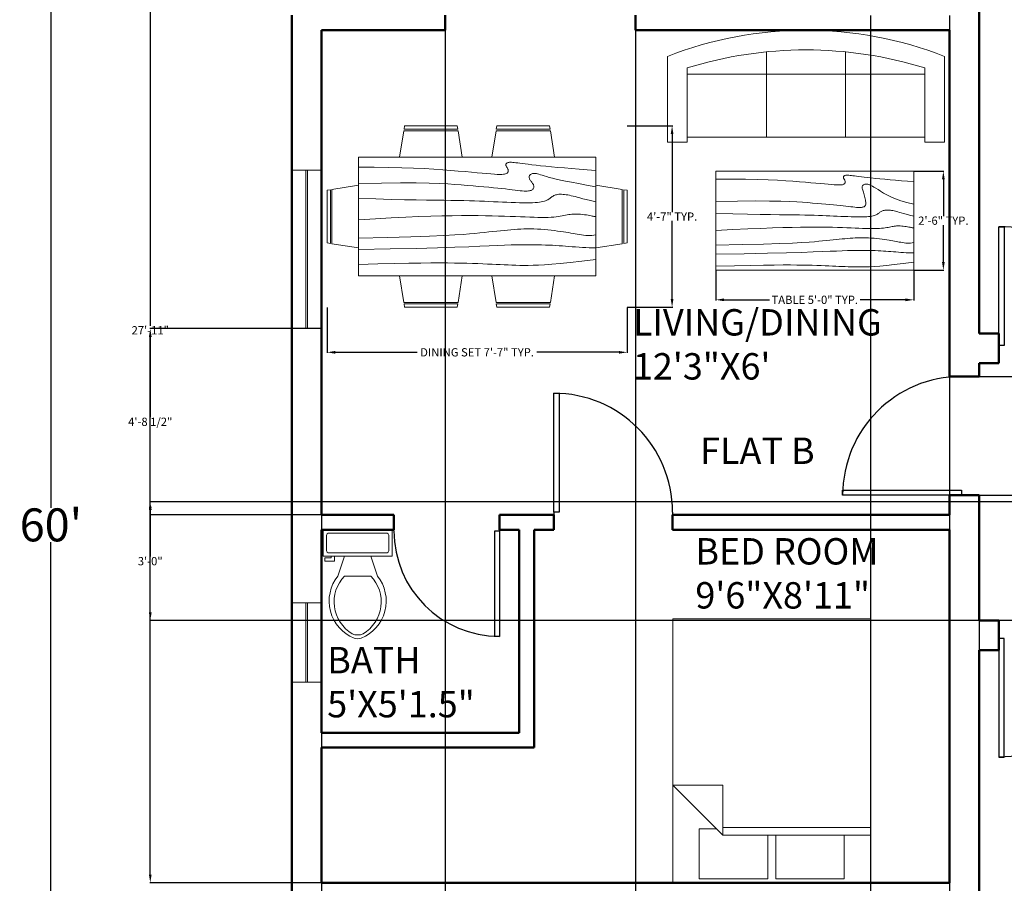
# Model space of a CAD drawing. Units: inches. Extents: x -46 to 565, y -56 to 809.
# Tile 3 of 6: x -46 to 252, y 296 to 557. Entities that reach past the tile are written whole.
import ezdxf

# ---------------------------------------------------------------- set-up
doc = ezdxf.new("R2010")
doc.units = ezdxf.units.IN
doc.header["$MEASUREMENT"] = 0
for name, color, linetype, lineweight in [('A-ANNO-DIMS', 2, 'Continuous', 18), ('A-AREA-IDEN', 241, 'Continuous', 18), ('A-FLOR-FIXT', 131, 'Continuous', 18), ('A-FURN', 131, 'Continuous', 18), ('DOOR', 210, 'Continuous', 25), ('WALL', 10, 'Continuous', 50), ('WINDOW', 170, 'Continuous', 18)]:
    doc.layers.add(name, color=color, linetype=linetype, lineweight=lineweight)
doc.styles.get("Standard").update_dxf_attribs({"font": 'arial.ttf'})
doc.dimstyles.get("Standard").update_dxf_attribs({"dimtxt": 2.5, "dimasz": 2.5, "dimexe": 0.18, "dimexo": 0.0625, "dimgap": 0.09, "dimtad": 0, "dimtih": 1, "dimtoh": 1, "dimzin": 0, "dimdsep": 46, "dimlunit": 3, "dimtxsty": 'Standard', "dimcen": 0.09, "dimadec": 0, "dimazin": 0, "dimtfac": 1, "dimtofl": 0, "dimtmove": 0, "dimatfit": 3, "dimfxl": 1, "dimtolj": 1, "dimtzin": 0, "dimarcsym": 0})

# ---------------------------------------------------------------- blocks, each defined once
blk = doc.blocks.new('*U2')
for p, q in [((0, 0), (0, -6)), ((40, 0), (40, -6))]:
    blk.add_line(p, q)
blk.add_lwpolyline([(0, 0), (0, 40), (1.75, 40), (1.75, 0)], close=True)
blk.add_arc((0, 0), 40, 0, 90)
blk = doc.blocks.new('Bed - Queen')
for p, q in [((0, -80.00003), (0, 0)), ((0, 0), (59.99999, 0)), ((59.99999, 0), (59.99999, -80.00003)), ((7.99999, -1.2), (28.79998, -1.2)), ((7.99999, -14.4), (7.99999, -1.2)), ((28.79998, -1.2), (28.79998, -14.4)), ((31.19999, -1.2), (51.99999, -1.2)), ((31.19999, -14.4), (31.19999, -1.2)), ((51.99999, -1.2), (51.99999, -16.4)), ((0, -14.4), (44.8, -14.4)), ((59.99999, -29.6), (44.8, -14.4)), ((44.8, -14.4), (44.8, -29.6)), ((44.8, -16.8), (0, -16.8)), ((51.99999, -16.4), (46.79936, -16.4)), ((44.8, -29.6), (59.99999, -29.6)), ((59.99999, -80.00003), (0, -80.00003))]:
    blk.add_line(p, q)
blk = doc.blocks.new('Toilet - top')
for p, q in [((9.5, -6), (9.5, -2)), ((-10, -8.5), (-8, -8.5)), ((-10, -9.5), (-10, -8.5)), ((-8, -8.5), (-8, -8)), ((-7, -8), (-7, -9.5)), ((-4, -8), (-6, -14)), ((4, -8), (6, -14)), ((-7, -9.5), (-10, -9.5)), ((4, -14), (-4, -14))]:
    blk.add_line(p, q)
blk.add_lwpolyline([(10.5, -8), (10.5, 0), (-10.5, 0), (-10.5, -8)], close=True)
for points in [[(-9.5, -2), (-9.5, -6)], [(8.5, -1), (-8.5, -1)], [(-8.5, -7), (8.5, -7)]]:
    blk.add_lwpolyline(points)
for centre, radius, start, end in [((-8.62, -1.88), 0.884, 81.8699, 188.1301), ((8.62, -1.88), 0.884, 351.8699, 98.1301), ((-8.62, -6.12), 0.884, 171.8699, 278.1301), ((8.62, -6.12), 0.884, 261.8699, 8.1301), ((3.52, -21.58), 12.17, 141.4691, 247.9714), ((4.2, -21.82), 11.33, 136.3677, 238.9468), ((-3.52, -21.58), 12.17, 292.0284, 38.5307), ((-4.2, -21.82), 11.33, 301.053, 43.6321), ((0, -27.88), 4, 245.7318, 294.2682), ((0, -29), 4, 254.8605, 285.1395)]:
    blk.add_arc(centre, radius, start, end)
blk = doc.blocks.new('Dining Set - 36 x 72 in.')
for p, q in [((-22, 27.5), (-22.1562, 26.50042)), ((-22, 27.5), (-6, 27.5)), ((-5.8437, 26.49966), (-6, 27.5)), ((6, 27.5), (5.8438, 26.50042)), ((6, 27.5), (22, 27.5)), ((22.1563, 26.49966), (22, 27.5)), ((-22.2343, 26.00059), (-23.4847, 17.99762)), ((-22.2304, 26), (-5.7608, 26)), ((-5.8416, 26.5), (-22.1534, 26.5)), ((-4.5152, 17.99762), (-5.7655, 25.99926)), ((5.7657, 26.00059), (4.5153, 17.99762)), ((5.7696, 26), (22.2392, 26)), ((22.1584, 26.5), (5.8466, 26.5)), ((23.4848, 17.99762), (22.2345, 25.99926)), ((36, 18), (-36, 18)), ((-36, 18), (-36, -18)), ((36, -18), (36, 18)), ((-44.0006, 8.23428), (-35.9976, 9.48474)), ((44.0006, 8.23428), (35.9976, 9.48474)), ((-45.5, 8), (-44.5004, 8.15617)), ((-45.5, 8), (-45.5, -8)), ((-44.5, -8.15843), (-44.5, 8.15338)), ((-44, 8.23041), (-44, -8.23915)), ((44, 8.23041), (44, -8.23915)), ((44.5, -8.15843), (44.5, 8.15338)), ((45.5, 8), (44.5005, 8.15617)), ((45.5, 8), (45.5, -8)), ((-44.4997, -8.15631), (-45.5, -8)), ((-35.9976, -9.48476), (-43.9993, -8.2345)), ((35.9976, -9.48476), (43.9993, -8.2345)), ((44.4997, -8.15631), (45.5, -8)), ((-36, -18), (36, -18)), ((-22.2343, -26.0006), (-23.4847, -17.99762)), ((-4.5152, -17.99762), (-5.7655, -25.99928)), ((5.7657, -26.0006), (4.5153, -17.99762)), ((23.4848, -17.99762), (22.2345, -25.99928)), ((-22.2304, -26), (-5.7608, -26)), ((-22, -27.5), (-22.1562, -26.50044)), ((-5.8416, -26.5), (-22.1534, -26.5)), ((-5.8437, -26.49967), (-6, -27.5)), ((5.7696, -26), (22.2392, -26)), ((6, -27.5), (5.8438, -26.50044)), ((22.1584, -26.5), (5.8466, -26.5)), ((22.1563, -26.49967), (22, -27.5)), ((-22, -27.5), (-6, -27.5)), ((6, -27.5), (22, -27.5))]:
    blk.add_line(p, q)
for points in [[(-36, 15), (-31.1772, 14.97754), (-26.8079, 14.91406), (-22.8538, 14.81543), (-19.276, 14.6875), (-16.0362, 14.53613), (-13.0957, 14.36718), (-10.4159, 14.18652), (-7.9583, 14), (-5.6904, 13.81315), (-3.6035, 13.63021), (-1.6954, 13.45508), (0.0365, 13.29166), (1.5945, 13.14388), (2.9811, 13.01562), (4.1988, 12.9108), (5.25, 12.83333), (6.1393, 12.78613), (6.8802, 12.76823), (7.4883, 12.77767), (7.9792, 12.8125), (8.3685, 12.87077), (8.6719, 12.95052), (8.9049, 13.0498), (9.0833, 13.16666), (9.2205, 13.29899), (9.3216, 13.44401), (9.3895, 13.59879), (9.4271, 13.76041), (9.4373, 13.92594), (9.4232, 14.09245), (9.3875, 14.257), (9.3333, 14.41666), (9.2638, 14.56917), (9.1836, 14.71484), (9.0975, 14.85465), (9.0104, 14.98958), (8.9272, 15.1206), (8.8529, 15.2487), (8.7922, 15.37483), (8.75, 15.5), (8.7305, 15.62467), (8.7344, 15.74739), (8.7617, 15.86621), (8.8125, 15.97916), (8.8867, 16.08431), (8.9844, 16.17968), (9.1055, 16.26334), (9.25, 16.33333), (9.4189, 16.38802), (9.6172, 16.42708), (9.8506, 16.45052), (10.125, 16.45833), (10.4463, 16.45052), (10.8203, 16.42708), (11.2529, 16.38802), (11.75, 16.33333), (12.3184, 16.26318), (12.9694, 16.17838), (13.7151, 16.07991), (14.5677, 15.96875), (15.5395, 15.84586), (16.6426, 15.71224), (17.8893, 15.56884), (19.2917, 15.41666), (20.859, 15.25667), (22.5879, 15.08984), (24.4721, 14.91715), (26.5052, 14.73958), (28.6809, 14.5581), (30.9929, 14.3737), (33.4347, 14.18733), (36, 14)], [(-36, 10), (-28.9766, 10.14274), (-23.1725, 10.20442), (-18.4241, 10.19775), (-14.5677, 10.13541), (-11.4399, 10.03011), (-8.877, 9.89453), (-6.7154, 9.74137), (-4.7917, 9.58333), (-2.9698, 9.43082), (-1.2246, 9.28515), (0.4415, 9.14534), (2.026, 9.01041), (3.5266, 8.87939), (4.9408, 8.7513), (6.266, 8.62516), (7.5, 8.5), (8.6411, 8.37549), (9.6914, 8.2539), (10.6538, 8.13818), (11.5312, 8.03125), (12.3267, 7.93603), (13.043, 7.85547), (13.6831, 7.79248), (14.25, 7.75), (14.7471, 7.7303), (15.1797, 7.73307), (15.5537, 7.75732), (15.875, 7.80208), (16.1494, 7.86637), (16.3828, 7.94922), (16.5811, 8.04964), (16.75, 8.16666), (16.8944, 8.29915), (17.0143, 8.44531), (17.1089, 8.60319), (17.1771, 8.77083), (17.218, 8.94629), (17.2305, 9.1276), (17.2137, 9.31282), (17.1667, 9.5), (17.0895, 9.6875), (16.987, 9.875), (16.8649, 10.0625), (16.7292, 10.25), (16.5856, 10.4375), (16.4401, 10.625), (16.2985, 10.8125), (16.1667, 11), (16.05, 11.18733), (15.9518, 11.3737), (15.8752, 11.5581), (15.8229, 11.73958), (15.798, 11.91715), (15.8034, 12.08984), (15.842, 12.25667), (15.9167, 12.41666), (16.0295, 12.56836), (16.1784, 12.70833), (16.3605, 12.83268), (16.5729, 12.9375), (16.8127, 13.01888), (17.0768, 13.07291), (17.3625, 13.0957), (17.6667, 13.08333), (17.9894, 13.03312), (18.3418, 12.94726), (18.7382, 12.82918), (19.1927, 12.68229), (19.7195, 12.51001), (20.3327, 12.31575), (21.0465, 12.10294), (21.875, 11.875), (22.8357, 11.63354), (23.959, 11.37304), (25.2786, 11.08618), (26.8282, 10.76562), (28.6414, 10.40405), (30.752, 9.99414), (33.1936, 9.52856), (36, 9)], [(-36, 5.5), (-30.7157, 5.3348), (-26.069, 5.20963), (-21.9946, 5.11767), (-18.4271, 5.05208), (-15.3009, 5.00602), (-12.5508, 4.97265), (-10.1112, 4.94515), (-7.9167, 4.91666), (-5.909, 4.88167), (-4.0586, 4.83984), (-2.3429, 4.79215), (-0.7396, 4.73958), (0.7739, 4.6831), (2.22, 4.6237), (3.6213, 4.56233), (5, 4.5), (6.373, 4.43782), (7.7344, 4.3776), (9.0723, 4.32129), (10.375, 4.27083), (11.6309, 4.22819), (12.8281, 4.19531), (13.9551, 4.17415), (15, 4.16666), (15.954, 4.17448), (16.819, 4.19791), (17.6001, 4.23698), (18.3021, 4.29166), (18.9299, 4.36198), (19.4883, 4.44791), (19.9823, 4.54948), (20.4167, 4.66666), (20.7969, 4.79899), (21.1302, 4.94401), (21.4245, 5.09879), (21.6875, 5.26041), (21.9271, 5.42594), (22.1511, 5.59245), (22.3672, 5.757), (22.5834, 5.91666), (22.8065, 6.06868), (23.0404, 6.21093), (23.2879, 6.34147), (23.5521, 6.45833), (23.8358, 6.55957), (24.142, 6.64323), (24.4735, 6.70735), (24.8334, 6.75), (25.2235, 6.76969), (25.642, 6.76692), (26.0858, 6.74267), (26.5521, 6.69791), (27.0379, 6.63362), (27.5404, 6.55078), (28.0565, 6.45036), (28.5834, 6.33333), (29.1242, 6.19987), (29.7071, 6.04687), (30.3661, 5.87044), (31.1354, 5.66666), (32.0493, 5.43164), (33.142, 5.16146), (34.4475, 4.85221), (36, 4.5)], [(-36, -1), (-30.7915, -0.6591), (-26.0195, -0.38216), (-21.6519, -0.16284), (-17.6563, 0.00521), (-14.0005, 0.12833), (-10.6523, 0.21289), (-7.5796, 0.26522), (-4.75, 0.29166), (-2.134, 0.29793), (0.2878, 0.28711), (2.5317, 0.26163), (4.6146, 0.22396), (6.5529, 0.17651), (8.3633, 0.12174), (10.0623, 0.06209), (11.6667, 0), (13.1899, -0.06201), (14.6341, -0.1211), (15.9982, -0.17432), (17.2813, -0.21875), (18.4823, -0.25147), (19.6003, -0.26953), (20.6343, -0.27002), (21.5834, -0.25), (22.4481, -0.20768), (23.2357, -0.14584), (23.9549, -0.06836), (24.6146, 0.02083), (25.2235, 0.11784), (25.7904, 0.21875), (26.3241, 0.31966), (26.8334, 0.41666), (27.3265, 0.50618), (27.8099, 0.58593), (28.2894, 0.65397), (28.7709, 0.70833), (29.2601, 0.74707), (29.763, 0.76823), (30.2855, 0.76985), (30.8334, 0.75), (31.4088, 0.70784), (31.9994, 0.64713), (32.589, 0.57275), (33.1615, 0.48958), (33.7008, 0.4025), (34.1908, 0.3164), (34.6153, 0.23616), (34.9584, 0.16666), (35.2099, 0.11165), (35.3848, 0.07031), (35.504, 0.04069), (35.5886, 0.02083), (35.6594, 0.00879), (35.7377, 0.0026), (35.8442, 0.00032), (36, 0)], [(-36, -6.5), (-27.1843, -6.31267), (-20.084, -6.1263), (-14.469, -5.9419), (-10.1094, -5.76042), (-6.7752, -5.58285), (-4.2363, -5.41016), (-2.2629, -5.24333), (-0.625, -5.08334), (0.8708, -4.93099), (2.2715, -4.78646), (3.5872, -4.64974), (4.8281, -4.52084), (6.0046, -4.39974), (7.127, -4.28646), (8.2053, -4.18099), (9.25, -4.08334), (10.2705, -3.99382), (11.2734, -3.91407), (12.2647, -3.84603), (13.25, -3.79167), (14.2354, -3.75293), (15.2266, -3.73177), (16.2295, -3.73015), (17.25, -3.75), (18.2912, -3.79248), (19.3451, -3.85547), (20.4009, -3.93604), (21.4479, -4.03125), (22.4754, -4.13819), (23.4727, -4.25391), (24.4289, -4.37549), (25.3334, -4.5), (26.1785, -4.62492), (26.9694, -4.74935), (27.7145, -4.87281), (28.4219, -4.99479), (29.1, -5.11483), (29.7572, -5.23242), (30.4016, -5.34709), (31.0417, -5.45834), (31.6837, -5.56437), (32.3262, -5.65821), (32.9658, -5.73153), (33.599, -5.77604), (34.2224, -5.78345), (34.8327, -5.74545), (35.4264, -5.65373), (36, -5.5)], [(-36, -10), (-26.4022, -9.81299), (-18.4675, -9.62891), (-11.9839, -9.45069), (-6.7396, -9.28125), (-2.5226, -9.12354), (0.8789, -8.98047), (3.6769, -8.85498), (6.0833, -8.75), (8.2767, -8.66765), (10.3021, -8.60677), (12.1712, -8.56543), (13.8958, -8.54167), (15.4876, -8.53353), (16.9583, -8.53907), (18.3197, -8.55632), (19.5834, -8.58334), (20.7616, -8.61841), (21.8685, -8.66081), (22.9188, -8.71004), (23.9271, -8.76563), (24.9081, -8.82707), (25.8763, -8.89388), (26.8465, -8.96558), (27.8334, -9.04167), (28.8474, -9.12118), (29.8828, -9.20117), (30.93, -9.27824), (31.9792, -9.34896), (33.0205, -9.40991), (34.0443, -9.45768), (35.0407, -9.48885), (36, -9.5)], [(-36, -14.5), (-30.0881, -14.33513), (-25.0332, -14.21224), (-20.7312, -14.12647), (-17.0781, -14.07292), (-13.97, -14.04671), (-11.3027, -14.04297), (-8.9724, -14.05681), (-6.875, -14.08334), (-4.9224, -14.11833), (-3.0905, -14.16016), (-1.3709, -14.20785), (0.2448, -14.26042), (1.7647, -14.3169), (3.1973, -14.3763), (4.5507, -14.43767), (5.8333, -14.5), (7.0554, -14.5621), (8.235, -14.62175), (9.3922, -14.67652), (10.5469, -14.72396), (11.7192, -14.76164), (12.929, -14.78711), (14.1965, -14.79794), (15.5417, -14.79167), (16.9933, -14.76424), (18.6152, -14.70508), (20.4804, -14.60197), (22.6615, -14.44271), (25.2312, -14.21509), (28.2624, -13.9069), (31.8277, -13.50594), (36, -13)]]:
    blk.add_lwpolyline(points)
blk = doc.blocks.new('Sofa - Roundback 7 ft.')
for p, q in [((-12.00002, -32.4421), (-12.00003, -6.5971)), ((11.99997, -32.4421), (11.99998, -6.5971)), ((-36.000027, -34), (-36.000027, -11.4696)), ((35.99998, -34), (35.99998, -11.4696)), ((-35.999844, -13.3819), (35.9998, -13.3819)), ((-36.000027, -32.4421), (35.99998, -32.4421))]:
    blk.add_line(p, q)
for points in [[(-36.000027, -34), (-42.000027, -34), (-42.000027, -8)], [(41.99998, -8), (41.99998, -34), (35.99998, -34)]]:
    blk.add_lwpolyline(points)
for centre, radius, start, end in [((0, -114.25), 114.25, 68.43141, 111.5686), ((-0.00001, -127.1968), 121.1968, 72.72033, 107.2797)]:
    blk.add_arc(centre, radius, start, end)
blk = doc.blocks.new('Table - Rectangular Woodgrain 60 x 30 in.')
for p, q in [((0, 0), (0, -30)), ((60, 0), (0, 0)), ((60, -30), (60, 0)), ((0, -30), (60, -30))]:
    blk.add_line(p, q)
for points in [[(0, -2.4), (4.8155, -2.418), (9.0302, -2.4688), (12.709, -2.5477), (15.9167, -2.65), (18.7181, -2.7711), (21.1781, -2.9063), (23.3616, -3.0508), (25.3333, -3.2), (27.1477, -3.3495), (28.8172, -3.4958), (30.3437, -3.636), (31.7291, -3.7667), (32.9756, -3.8849), (34.0849, -3.9875), (35.059, -4.0714), (35.9, -4.1334), (36.6114, -4.1711), (37.2041, -4.1854), (37.6906, -4.1779), (38.0833, -4.15), (38.3948, -4.1034), (38.6375, -4.0396), (38.8239, -3.9602), (38.9666, -3.8667), (39.0764, -3.7608), (39.1573, -3.6448), (39.2116, -3.521), (39.2416, -3.3917), (39.2498, -3.2593), (39.2385, -3.1261), (39.21, -2.9944), (39.1666, -2.8667), (39.111, -2.7447), (39.0468, -2.6281), (38.978, -2.5163), (38.9083, -2.4083), (38.8418, -2.3035), (38.7823, -2.201), (38.7337, -2.1001), (38.7, -2), (38.6844, -1.9003), (38.6875, -1.8021), (38.7094, -1.707), (38.75, -1.6167), (38.8094, -1.5326), (38.8875, -1.4563), (38.9844, -1.3893), (39.1, -1.3333), (39.2351, -1.2896), (39.3937, -1.2583), (39.5804, -1.2396), (39.8, -1.2333), (40.057, -1.2396), (40.3562, -1.2583), (40.7023, -1.2896), (41.1, -1.3333), (41.5547, -1.3895), (42.0755, -1.4573), (42.6721, -1.5361), (43.3542, -1.625), (44.1316, -1.7233), (45.014, -1.8302), (46.0114, -1.9449), (47.1333, -2.0667), (48.3862, -2.1947), (49.7625, -2.3281), (51.2513, -2.4663), (52.8416, -2.6083), (54.5226, -2.7535), (56.2833, -2.9011), (58.1127, -3.0501), (60, -3.2)], [(0, -9.2), (6.5759, -9.0858), (11.9385, -9.0365), (16.2527, -9.0418), (19.6833, -9.0917), (22.3952, -9.1759), (24.5531, -9.2844), (26.322, -9.4069), (27.8666, -9.5333), (29.3241, -9.6553), (30.7203, -9.7719), (32.0532, -9.8837), (33.3208, -9.9917), (34.5213, -10.0965), (35.6526, -10.199), (36.7128, -10.2999), (37.7, -10.4), (38.6129, -10.4996), (39.4531, -10.5969), (40.223, -10.6895), (40.925, -10.775), (41.5613, -10.8512), (42.1344, -10.9156), (42.6465, -10.966), (43.1, -11), (43.4976, -11.0158), (43.8437, -11.0136), (44.143, -10.9942), (44.4, -10.9583), (44.6195, -10.9069), (44.8062, -10.8406), (44.9648, -10.7603), (45.1, -10.6667), (45.2155, -10.5598), (45.3114, -10.4365), (45.3871, -10.2929), (45.4416, -10.125), (45.4743, -9.929), (45.4844, -9.7011), (45.4709, -9.4371), (45.4333, -9.1333), (45.3716, -8.7883), (45.2896, -8.4104), (45.1919, -8.0107), (45.0833, -7.6), (44.9685, -7.1893), (44.8521, -6.7896), (44.7388, -6.4117), (44.6333, -6.0667), (44.54, -5.7628), (44.4614, -5.4979), (44.4001, -5.2675), (44.3583, -5.0667), (44.3384, -4.8909), (44.3427, -4.7354), (44.3736, -4.5956), (44.4333, -4.4667), (44.5236, -4.3453), (44.6427, -4.2333), (44.7884, -4.1339), (44.9583, -4.05), (45.1501, -3.9849), (45.3614, -3.9417), (45.59, -3.9234), (45.8333, -3.9333), (46.0915, -3.9749), (46.3734, -4.0531), (46.6906, -4.1736), (47.0542, -4.3417), (47.4756, -4.5629), (47.9661, -4.8427), (48.5372, -5.1866), (49.2, -5.6), (49.9676, -6.0844), (50.8594, -6.625), (51.8965, -7.2031), (53.1, -7.8), (54.491, -8.3969), (56.0906, -8.975), (57.9199, -9.5156), (60, -10)], [(0, -12.8), (5.1847, -12.9322), (9.6213, -13.0323), (13.3963, -13.1059), (16.5958, -13.1583), (19.3063, -13.1952), (21.614, -13.2219), (23.6054, -13.2439), (25.3666, -13.2667), (26.9728, -13.2947), (28.4531, -13.3281), (29.8256, -13.3663), (31.1083, -13.4083), (32.3191, -13.4535), (33.476, -13.501), (34.597, -13.5501), (35.7, -13.6), (36.7984, -13.6497), (37.8875, -13.6979), (38.9578, -13.743), (40, -13.7833), (41.0047, -13.8174), (41.9625, -13.8438), (42.864, -13.8607), (43.7, -13.8667), (44.4631, -13.8604), (45.1552, -13.8417), (45.7801, -13.8104), (46.3416, -13.7667), (46.8439, -13.7104), (47.2906, -13.6417), (47.6858, -13.5604), (48.0333, -13.4667), (48.3375, -13.3608), (48.6042, -13.2448), (48.8396, -13.121), (49.05, -12.9917), (49.2417, -12.8593), (49.4208, -12.7261), (49.5937, -12.5944), (49.7667, -12.4667), (49.9452, -12.3451), (50.1323, -12.2313), (50.3303, -12.1268), (50.5416, -12.0333), (50.7686, -11.9524), (51.0135, -11.8854), (51.2788, -11.8341), (51.5666, -11.8), (51.8785, -11.7843), (52.2116, -11.7865), (52.562, -11.8059), (52.926, -11.8417), (53.2998, -11.8931), (53.6795, -11.9594), (54.0614, -12.0397), (54.4416, -12.1333), (54.8223, -12.2401), (55.2293, -12.3625), (55.6942, -12.5037), (56.2489, -12.6667), (56.9251, -12.8547), (57.7545, -13.0708), (58.7689, -13.3182), (60, -13.6)], [(0, -18), (5.124, -17.7273), (9.6609, -17.5057), (13.6705, -17.3303), (17.2125, -17.1958), (20.3467, -17.0973), (23.1328, -17.0297), (25.6307, -16.9878), (27.9, -16.9667), (29.9928, -16.9617), (31.9302, -16.9703), (33.7254, -16.9907), (35.3917, -17.0208), (36.9423, -17.0588), (38.3906, -17.1026), (39.7499, -17.1503), (41.0333, -17.2), (42.2519, -17.2496), (43.4073, -17.2969), (44.4986, -17.3395), (45.525, -17.375), (46.4858, -17.4012), (47.3802, -17.4156), (48.2074, -17.416), (48.9667, -17.4), (49.6583, -17.3662), (50.2872, -17.3167), (50.8595, -17.2547), (51.3812, -17.1833), (51.8584, -17.1057), (52.2971, -17.025), (52.7034, -16.9443), (53.0833, -16.8667), (53.443, -16.7951), (53.789, -16.7313), (54.128, -16.6768), (54.4666, -16.6334), (54.8115, -16.6024), (55.1693, -16.5854), (55.5465, -16.5841), (55.95, -16.6), (56.3828, -16.6337), (56.8346, -16.6823), (57.2915, -16.7418), (57.7396, -16.8084), (58.165, -16.878), (58.5539, -16.9469), (58.8924, -17.0111), (59.1666, -17.0667), (59.3679, -17.1107), (59.5078, -17.1438), (59.6032, -17.1675), (59.6708, -17.1833), (59.7275, -17.193), (59.7901, -17.1979), (59.8753, -17.1998), (60, -17.2)], [(0, -22.4), (8.0098, -22.2501), (14.4094, -22.1011), (19.4168, -21.9535), (23.25, -21.8083), (26.1269, -21.6663), (28.2656, -21.5281), (29.884, -21.3947), (31.2, -21.2667), (32.3967, -21.1448), (33.5172, -21.0292), (34.5697, -20.9198), (35.5625, -20.8167), (36.5037, -20.7198), (37.4015, -20.6292), (38.2642, -20.5448), (39.1, -20.4667), (39.9164, -20.3951), (40.7187, -20.3313), (41.5117, -20.2768), (42.3, -20.2333), (43.0883, -20.2024), (43.8812, -20.1854), (44.6836, -20.1841), (45.5, -20.2), (46.3328, -20.234), (47.1747, -20.2844), (48.0163, -20.3488), (48.8479, -20.425), (49.66, -20.5106), (50.4429, -20.6031), (51.1872, -20.7004), (51.8833, -20.8), (52.5246, -20.8999), (53.1166, -20.9995), (53.6681, -21.0983), (54.1875, -21.1958), (54.6834, -21.2919), (55.1646, -21.3859), (55.6394, -21.4777), (56.1167, -21.5667), (56.6028, -21.6515), (57.0961, -21.7266), (57.5929, -21.7852), (58.0896, -21.8208), (58.5823, -21.8268), (59.0674, -21.7964), (59.5412, -21.723), (60, -21.6)], [(0, -25.2), (8.6355, -25.0504), (15.7026, -24.9031), (21.4049, -24.7606), (25.9458, -24.625), (29.529, -24.4988), (32.3578, -24.3844), (34.6359, -24.284), (36.5667, -24.2), (38.3213, -24.1341), (39.9417, -24.0854), (41.437, -24.0523), (42.8167, -24.0333), (44.0901, -24.0268), (45.2667, -24.0313), (46.3557, -24.0451), (47.3667, -24.0667), (48.309, -24.0947), (49.1928, -24.1287), (50.0284, -24.168), (50.826, -24.2125), (51.5959, -24.2617), (52.3483, -24.3151), (53.0935, -24.3725), (53.8417, -24.4334), (54.6009, -24.497), (55.3699, -24.561), (56.1454, -24.6226), (56.9239, -24.6792), (57.7021, -24.7279), (58.4764, -24.7662), (59.2435, -24.7911), (60, -24.8)], [(0, -28.8), (5.6867, -28.6681), (10.45, -28.5698), (14.407, -28.5012), (17.675, -28.4584), (20.3711, -28.4374), (22.6125, -28.4344), (24.5164, -28.4455), (26.2, -28.4667), (27.762, -28.4947), (29.2276, -28.5281), (30.6033, -28.5663), (31.8958, -28.6084), (33.1118, -28.6535), (34.2578, -28.7011), (35.3405, -28.7501), (36.3666, -28.8), (37.3443, -28.8497), (38.288, -28.8974), (39.2137, -28.9412), (40.1375, -28.9792), (41.0753, -29.0093), (42.0432, -29.0297), (43.0572, -29.0384), (44.1333, -29.0333), (45.2936, -29.0114), (46.5843, -28.9641), (48.0579, -28.8816), (49.7666, -28.7542), (51.7629, -28.5721), (54.0989, -28.3255), (56.8272, -28.0048), (60, -27.6)]]:
    blk.add_lwpolyline(points)
blk = doc.blocks.new('*D15')
at = {"layer": 'A-ANNO-DIMS', "color": 0, "lineweight": -2, "transparency": 16777216}
for p, q in [((174.08, 764.2), (-37.07, 764.2)), ((-36.89, 761.7), (-36.89, 409.4)), ((-36.89, 46.7), (-36.89, 399)), ((174.08, 44.2), (-37.07, 44.2))]:
    blk.add_line(p, q, dxfattribs=at)
at = {"layer": 'A-ANNO-DIMS', "color": 0, "transparency": 16777216}
for points in [[(-37.31, 761.7), (-36.48, 761.7), (-36.89, 764.2)], [(-37.31, 46.7), (-36.48, 46.7), (-36.89, 44.2)]]:
    blk.add_solid(points, dxfattribs=at)
at = {"layer": 'Defpoints', "color": 0, "transparency": 16777216}
for p in [(-36.89, 764.2), (174.14, 764.2), (174.14, 44.2)]:
    blk.add_point(p, dxfattribs=at)
at = {"layer": 'A-ANNO-DIMS', "color": 0, "transparency": 16777216, "insert": (-36.89, 404.2), "char_height": 10, "attachment_point": 5}
blk.add_mtext("\\A1;60'", dxfattribs=at)
blk = doc.blocks.new('WIN-48IN')
for p, q in [((0, 4.75), (48, 4.75)), ((0, 4.25), (48, 4.25))]:
    blk.add_line(p, q)
blk.add_lwpolyline([(0, 0), (48, 0), (48, 9), (0, 9)], close=True)
blk = doc.blocks.new('WIN-24IN')
for p, q in [((4.25, 24), (4.25, 0)), ((4.75, 24), (4.75, 0))]:
    blk.add_line(p, q)
blk.add_lwpolyline([(0, 24), (0, 0), (9, 0), (9, 24)], close=True)
blk = doc.blocks.new('*D27')
at = {"layer": 'A-ANNO-DIMS', "color": 0, "lineweight": -2, "transparency": 16777216}
for p, q in [((164.78, 481.37), (164.78, 472.25)), ((224.78, 481.37), (224.78, 472.25)), ((167.28, 472.43), (181.02, 472.43)), ((222.28, 472.43), (208.54, 472.43))]:
    blk.add_line(p, q, dxfattribs=at)
at = {"layer": 'A-ANNO-DIMS', "color": 0, "transparency": 16777216}
for points in [[(167.28, 472.85), (167.28, 472.02), (164.78, 472.43)], [(222.28, 472.85), (222.28, 472.02), (224.78, 472.43)]]:
    blk.add_solid(points, dxfattribs=at)
at = {"layer": 'Defpoints', "color": 0, "transparency": 16777216}
for p in [(164.78, 481.43), (224.78, 481.43), (224.78, 472.43)]:
    blk.add_point(p, dxfattribs=at)
at = {"layer": 'A-ANNO-DIMS', "color": 0, "transparency": 16777216, "insert": (194.78, 472.43), "char_height": 2.5, "attachment_point": 5}
blk.add_mtext('\\A1;TABLE 5\'-0" TYP.', dxfattribs=at)
blk = doc.blocks.new('*D28')
at = {"layer": 'A-ANNO-DIMS', "color": 0, "lineweight": -2, "transparency": 16777216}
for p, q in [((224.84, 511.43), (233.96, 511.43)), ((233.78, 508.93), (233.78, 497.8)), ((233.78, 483.93), (233.78, 495.07)), ((224.84, 481.43), (233.96, 481.43))]:
    blk.add_line(p, q, dxfattribs=at)
at = {"layer": 'A-ANNO-DIMS', "color": 0, "transparency": 16777216}
for points in [[(233.36, 508.93), (234.2, 508.93), (233.78, 511.43)], [(233.36, 483.93), (234.2, 483.93), (233.78, 481.43)]]:
    blk.add_solid(points, dxfattribs=at)
at = {"layer": 'Defpoints', "color": 0, "transparency": 16777216}
for p in [(224.78, 511.43), (233.78, 511.43), (224.78, 481.43)]:
    blk.add_point(p, dxfattribs=at)
at = {"layer": 'A-ANNO-DIMS', "color": 0, "transparency": 16777216, "insert": (233.78, 496.43), "char_height": 2.5, "attachment_point": 5}
blk.add_mtext('\\A1;2\'-6" TYP.', dxfattribs=at)
blk = doc.blocks.new('*D33')
at = {"layer": 'A-ANNO-DIMS', "color": 0, "lineweight": -2, "transparency": 16777216}
for p, q in [((46.86, 470.1), (46.86, 456.34)), ((137.86, 470.1), (137.86, 456.34)), ((49.36, 456.52), (74.23, 456.52)), ((135.36, 456.52), (110.48, 456.52))]:
    blk.add_line(p, q, dxfattribs=at)
at = {"layer": 'A-ANNO-DIMS', "color": 0, "transparency": 16777216}
for points in [[(49.36, 456.93), (49.36, 456.1), (46.86, 456.52)], [(135.36, 456.93), (135.36, 456.1), (137.86, 456.52)]]:
    blk.add_solid(points, dxfattribs=at)
at = {"layer": 'Defpoints', "color": 0, "transparency": 16777216}
for p in [(46.86, 470.17), (137.86, 470.17), (137.86, 456.52)]:
    blk.add_point(p, dxfattribs=at)
at = {"layer": 'A-ANNO-DIMS', "color": 0, "transparency": 16777216, "insert": (92.36, 456.52), "char_height": 2.5, "attachment_point": 5}
blk.add_mtext('\\A1;DINING SET 7\'-7" TYP.', dxfattribs=at)
blk = doc.blocks.new('*D34')
at = {"layer": 'A-ANNO-DIMS', "color": 0, "lineweight": -2, "transparency": 16777216}
for p, q in [((137.92, 525.17), (151.69, 525.17)), ((151.51, 522.67), (151.51, 499.01)), ((151.51, 472.67), (151.51, 496.33)), ((137.92, 470.17), (151.69, 470.17))]:
    blk.add_line(p, q, dxfattribs=at)
at = {"layer": 'A-ANNO-DIMS', "color": 0, "transparency": 16777216}
for points in [[(151.09, 522.67), (151.92, 522.67), (151.51, 525.17)], [(151.09, 472.67), (151.92, 472.67), (151.51, 470.17)]]:
    blk.add_solid(points, dxfattribs=at)
at = {"layer": 'Defpoints', "color": 0, "transparency": 16777216}
for p in [(137.86, 525.17), (151.51, 525.17), (137.86, 470.17)]:
    blk.add_point(p, dxfattribs=at)
at = {"layer": 'A-ANNO-DIMS', "color": 0, "transparency": 16777216, "insert": (151.51, 497.67), "char_height": 2.5, "attachment_point": 5}
blk.add_mtext('\\A1;4\'-7" TYP.', dxfattribs=at)
blk = doc.blocks.new('*D43')
at = {"layer": 'A-ANNO-DIMS', "color": 0, "lineweight": -2, "transparency": 16777216}
for p, q in [((244.64, 375.14), (244.64, 0.22)), ((351.14, 375.14), (351.14, 0.22)), ((247.14, 0.4), (290.59, 0.4)), ((348.64, 0.4), (305.19, 0.4))]:
    blk.add_line(p, q, dxfattribs=at)
at = {"layer": 'A-ANNO-DIMS', "color": 0, "transparency": 16777216}
for points in [[(247.14, 0.82), (247.14, -0.02), (244.64, 0.4)], [(348.64, 0.82), (348.64, -0.02), (351.14, 0.4)]]:
    blk.add_solid(points, dxfattribs=at)
at = {"layer": 'Defpoints', "color": 0, "transparency": 16777216}
for p in [(244.64, 375.2), (351.14, 375.2), (351.14, 0.4)]:
    blk.add_point(p, dxfattribs=at)
at = {"layer": 'A-ANNO-DIMS', "color": 0, "transparency": 16777216, "insert": (297.89, 0.4), "char_height": 2.5, "attachment_point": 5}
blk.add_mtext('\\A1;8\'-10 1/2"', dxfattribs=at)
blk = doc.blocks.new('*D44')
at = {"layer": 'A-ANNO-DIMS', "color": 0, "lineweight": -2, "transparency": 16777216}
for p, q in [((351.08, 411.2), (-6.94, 411.2)), ((-6.76, 408.7), (-6.76, 394.57)), ((-6.76, 377.7), (-6.76, 391.83)), ((351.08, 375.2), (-6.94, 375.2))]:
    blk.add_line(p, q, dxfattribs=at)
at = {"layer": 'A-ANNO-DIMS', "color": 0, "transparency": 16777216}
for points in [[(-7.17, 408.7), (-6.34, 408.7), (-6.76, 411.2)], [(-7.17, 377.7), (-6.34, 377.7), (-6.76, 375.2)]]:
    blk.add_solid(points, dxfattribs=at)
at = {"layer": 'Defpoints', "color": 0, "transparency": 16777216}
for p in [(-6.76, 411.2), (351.14, 411.2), (351.14, 375.2)]:
    blk.add_point(p, dxfattribs=at)
at = {"layer": 'A-ANNO-DIMS', "color": 0, "transparency": 16777216, "insert": (-6.76, 393.2), "char_height": 2.5, "attachment_point": 5}
blk.add_mtext('\\A1;3\'-0"', dxfattribs=at)
blk = doc.blocks.new('*D46')
at = {"layer": 'A-ANNO-DIMS', "color": 0, "lineweight": -2, "transparency": 16777216}
for p, q in [((36.08, 630.7), (-6.94, 630.7)), ((-6.76, 628.2), (-6.76, 464.54)), ((-6.76, 298.2), (-6.76, 461.85)), ((45.08, 295.7), (-6.94, 295.7))]:
    blk.add_line(p, q, dxfattribs=at)
at = {"layer": 'A-ANNO-DIMS', "color": 0, "transparency": 16777216}
for points in [[(-7.17, 628.2), (-6.34, 628.2), (-6.76, 630.7)], [(-7.17, 298.2), (-6.34, 298.2), (-6.76, 295.7)]]:
    blk.add_solid(points, dxfattribs=at)
at = {"layer": 'Defpoints', "color": 0, "transparency": 16777216}
for p in [(-6.76, 630.7), (36.14, 630.7), (45.14, 295.7)]:
    blk.add_point(p, dxfattribs=at)
at = {"layer": 'A-ANNO-DIMS', "color": 0, "transparency": 16777216, "insert": (-6.76, 463.2), "char_height": 2.5, "attachment_point": 5}
blk.add_mtext('\\A1;27\'-11"', dxfattribs=at)
blk = doc.blocks.new('*D50')
at = {"layer": 'A-ANNO-DIMS', "color": 0, "lineweight": -2, "transparency": 16777216}
for p, q in [((211.64, 558.64), (211.64, 0.22)), ((235.64, 558.64), (235.64, 0.22)), ((214.14, 0.4), (220.21, 0.4)), ((233.14, 0.4), (227.08, 0.4))]:
    blk.add_line(p, q, dxfattribs=at)
at = {"layer": 'A-ANNO-DIMS', "color": 0, "transparency": 16777216}
for points in [[(214.14, 0.82), (214.14, -0.02), (211.64, 0.4)], [(233.14, 0.82), (233.14, -0.02), (235.64, 0.4)]]:
    blk.add_solid(points, dxfattribs=at)
at = {"layer": 'Defpoints', "color": 0, "transparency": 16777216}
for p in [(211.64, 558.7), (235.64, 558.7), (235.64, 0.4)]:
    blk.add_point(p, dxfattribs=at)
at = {"layer": 'A-ANNO-DIMS', "color": 0, "transparency": 16777216, "insert": (223.64, 0.4), "char_height": 2.5, "attachment_point": 5}
blk.add_mtext('\\A1;2\'-0"', dxfattribs=at)
blk = doc.blocks.new('*D51')
at = {"layer": 'A-ANNO-DIMS', "color": 0, "lineweight": -2, "transparency": 16777216}
for p, q in [((82.64, 554.14), (82.64, 0.22)), ((140.42, 554.14), (140.42, 0.22)), ((85.14, 0.4), (107.1, 0.4)), ((137.92, 0.4), (115.96, 0.4))]:
    blk.add_line(p, q, dxfattribs=at)
at = {"layer": 'A-ANNO-DIMS', "color": 0, "transparency": 16777216}
for points in [[(85.14, 0.82), (85.14, -0.02), (82.64, 0.4)], [(137.92, 0.82), (137.92, -0.02), (140.42, 0.4)]]:
    blk.add_solid(points, dxfattribs=at)
at = {"layer": 'Defpoints', "color": 0, "transparency": 16777216}
for p in [(82.64, 554.2), (140.42, 554.2), (140.42, 0.4)]:
    blk.add_point(p, dxfattribs=at)
at = {"layer": 'A-ANNO-DIMS', "color": 0, "transparency": 16777216, "insert": (111.53, 0.4), "char_height": 2.5, "attachment_point": 5}
blk.add_mtext('\\A1;4\'-10"', dxfattribs=at)
blk = doc.blocks.new('*D53')
at = {"layer": 'A-ANNO-DIMS', "color": 0, "lineweight": -2, "transparency": 16777216}
for p, q in [((244.71, 449.2), (559.22, 449.2)), ((559.04, 446.7), (559.04, 432.57)), ((559.04, 415.7), (559.04, 429.83)), ((244.71, 413.2), (559.22, 413.2))]:
    blk.add_line(p, q, dxfattribs=at)
at = {"layer": 'A-ANNO-DIMS', "color": 0, "transparency": 16777216}
for points in [[(558.63, 446.7), (559.46, 446.7), (559.04, 449.2)], [(558.63, 415.7), (559.46, 415.7), (559.04, 413.2)]]:
    blk.add_solid(points, dxfattribs=at)
at = {"layer": 'Defpoints', "color": 0, "transparency": 16777216}
for p in [(244.64, 449.2), (559.04, 449.2), (244.64, 413.2)]:
    blk.add_point(p, dxfattribs=at)
at = {"layer": 'A-ANNO-DIMS', "color": 0, "transparency": 16777216, "insert": (559.04, 431.2), "char_height": 2.5, "attachment_point": 5}
blk.add_mtext('\\A1;3\'-0"', dxfattribs=at)
blk = doc.blocks.new('*D54')
at = {"layer": 'A-ANNO-DIMS', "color": 0, "lineweight": -2, "transparency": 16777216}
for p, q in [((45.08, 463.71), (-6.94, 463.71)), ((-6.76, 461.21), (-6.76, 436.84)), ((-6.76, 409.7), (-6.76, 434.07)), ((45.08, 407.2), (-6.94, 407.2))]:
    blk.add_line(p, q, dxfattribs=at)
at = {"layer": 'A-ANNO-DIMS', "color": 0, "transparency": 16777216}
for points in [[(-7.17, 461.21), (-6.34, 461.21), (-6.76, 463.71)], [(-7.17, 409.7), (-6.34, 409.7), (-6.76, 407.2)]]:
    blk.add_solid(points, dxfattribs=at)
at = {"layer": 'Defpoints', "color": 0, "transparency": 16777216}
for p in [(-6.76, 463.71), (45.14, 463.71), (45.14, 407.2)]:
    blk.add_point(p, dxfattribs=at)
at = {"layer": 'A-ANNO-DIMS', "color": 0, "transparency": 16777216, "insert": (-6.76, 435.46), "char_height": 2.5, "attachment_point": 5}
blk.add_mtext('\\A1;4\'-8 1/2"', dxfattribs=at)
blk = doc.blocks.new('*D55')
at = {"layer": 'A-ANNO-DIMS', "color": 0, "lineweight": -2, "transparency": 16777216}
for p, q in [((45.14, 407.14), (45.14, 0.22)), ((235.64, 407.14), (235.64, 0.22)), ((47.64, 0.4), (132.24, 0.4)), ((233.14, 0.4), (148.54, 0.4))]:
    blk.add_line(p, q, dxfattribs=at)
at = {"layer": 'A-ANNO-DIMS', "color": 0, "transparency": 16777216}
for points in [[(47.64, 0.82), (47.64, -0.02), (45.14, 0.4)], [(233.14, 0.82), (233.14, -0.02), (235.64, 0.4)]]:
    blk.add_solid(points, dxfattribs=at)
at = {"layer": 'Defpoints', "color": 0, "transparency": 16777216}
for p in [(45.14, 407.2), (235.64, 407.2), (235.64, 0.4)]:
    blk.add_point(p, dxfattribs=at)
at = {"layer": 'A-ANNO-DIMS', "color": 0, "transparency": 16777216, "insert": (140.39, 0.4), "char_height": 2.5, "attachment_point": 5}
blk.add_mtext('\\A1;15\'-10 1/2"', dxfattribs=at)

msp = doc.modelspace()

# ---------------------------------------------------------------- linework, layer by layer
at = {"layer": 'WALL'}
for p, q in [((244.643, 635.2), (244.643, 462.2)), ((36.143, 558.7), (36.143, 402.7)), ((82.643, 558.7), (82.643, 554.2)), ((140.418, 558.7), (140.418, 554.2)), ((45.143, 554.2), (45.143, 407.2)), ((82.643, 554.2), (45.143, 554.2)), ((235.643, 554.2), (140.418, 554.2)), ((235.643, 554.2), (235.643, 449.2)), ((250.643, 462.2), (244.643, 462.2)), ((250.643, 462.2), (250.643, 453.2)), ((250.643, 453.2), (244.643, 453.2)), ((244.643, 453.2), (244.643, 449.2)), ((235.643, 449.2), (244.643, 449.2)), ((235.643, 413.2), (244.643, 413.2)), ((235.643, 413.2), (235.643, 407.2)), ((244.643, 413.2), (244.643, 375.2)), ((67.143, 407.2), (45.143, 407.2)), ((67.143, 402.7), (67.143, 407.2)), ((99.143, 402.7), (99.143, 407.2)), ((115.643, 407.2), (99.143, 407.2)), ((115.643, 402.7), (115.643, 407.2)), ((235.643, 407.2), (151.643, 407.2)), ((151.643, 402.7), (151.643, 407.2)), ((36.143, 402.7), (36.143, 295.7)), ((45.143, 402.7), (45.143, 341.2)), ((67.143, 402.7), (45.143, 402.7)), ((105.143, 402.7), (99.143, 402.7)), ((105.143, 402.7), (105.143, 341.2)), ((109.643, 402.7), (109.643, 336.7)), ((115.643, 402.7), (109.643, 402.7)), ((235.643, 402.7), (151.643, 402.7)), ((235.643, 402.7), (235.643, 295.7)), ((250.643, 375.2), (244.643, 375.2)), ((250.643, 375.2), (250.643, 366.2)), ((250.643, 366.2), (244.643, 366.2)), ((244.643, 366.2), (244.643, 286.7)), ((105.143, 341.2), (45.143, 341.2)), ((109.643, 336.7), (45.143, 336.7)), ((45.143, 336.7), (45.143, 295.7)), ((36.143, 295.7), (36.143, 86.684)), ((235.643, 295.7), (45.143, 295.7))]:
    msp.add_line(p, q, dxfattribs=at)

# ---------------------------------------------------------------- block references
at = {"layer": 'A-FLOR-FIXT'}
msp.add_blockref('Toilet - top', (56.143, 402.7), dxfattribs=at)
at = {"layer": 'A-FURN'}
for name, p in [('Sofa - Roundback 7 ft.', (192.118, 554.2)), ('Dining Set - 36 x 72 in.', (92.356, 497.667)), ('Table - Rectangular Woodgrain 60 x 30 in.', (164.78, 511.432))]:
    msp.add_blockref(name, p, dxfattribs=at)
at = {"layer": 'A-FURN', "rotation": 180}
msp.add_blockref('Bed - Queen', (211.735, 295.7), dxfattribs=at)
at = {"layer": 'DOOR', "xscale": 0.9, "yscale": 0.9, "zscale": 0.9}
for p in [(250.643, 458.6), (115.643, 408.1)]:
    msp.add_blockref('*U2', p, dxfattribs=at)
at = {"layer": 'DOOR'}
for p, xscale, yscale, zscale, rotation in [((239.243, 413.2), 0.9, 0.9, 0.9, 90), ((99.143, 402.4), 0.8, 0.8, 0.8, 180), ((250.643, 369.8), -0.9000000000000007, 0.9000000000000007, 0.9000000000000007, 180)]:
    msp.add_blockref('*U2', p, dxfattribs=dict(at, xscale=xscale, yscale=yscale, zscale=zscale, rotation=rotation))
at = {"layer": 'WINDOW', "rotation": 269.9999999999999}
msp.add_blockref('WIN-48IN', (36.143, 511.712), dxfattribs=at)
at = {"layer": 'WINDOW'}
msp.add_blockref('WIN-24IN', (36.143, 356.537), dxfattribs=at)

# ---------------------------------------------------------------- texts
at = {"layer": 'A-AREA-IDEN', "char_height": 8, "attachment_point": 1}
for s, heights, insert in [('LIVING/DINING\\P12\'3"X6\'', [21.644], (139.623, 469.604)), ('FLAT B', [0], (160.013, 430.676)), ('BED ROOM\\P9\'6"X8\'11" ', [0], (158.568, 400.184)), ('BATH\\P5\'X5\'1.5"', [0], (46.906, 367.187))]:
    msp.add_mtext_dynamic_manual_height_columns(s, width=70.77133, gutter_width=1, heights=heights, dxfattribs=dict(at, insert=insert))

# ---------------------------------------------------------------- dimensions: what is measured, and where the dimension line sits
at = {"layer": 'A-ANNO-DIMS'}
dim = msp.add_aligned_dim(p1=(174.143, 44.2), p2=(174.143, 764.2), distance=211.037, dimstyle='Standard', override={"dimtxt": 10, "dimclrd": 0, "dimclre": 0, "dimclrt": 0}, dxfattribs=at)
dim.commit()
dim.dimension.update_dxf_attribs({"geometry": '*D15', "text_midpoint": (-36.894, 404.2)})
for base, p1, p2, picture, middle in [((-6.757, 630.7), (45.143, 295.7), (36.143, 630.7), '*D46', (-6.757, 463.2)), ((-6.757, 463.712), (45.143, 407.2), (45.143, 463.712), '*D54', (-6.757, 435.456)), ((559.043, 449.2), (244.643, 413.2), (244.643, 449.2), '*D53', (559.043, 431.2)), ((-6.757, 411.2), (351.143, 375.2), (351.143, 411.2), '*D44', (-6.757, 393.2))]:
    dim = msp.add_linear_dim(base=base, p1=p1, p2=p2, angle=90, dimstyle='Standard', override={"dimdec": 1, "dimlfac": 1, "dimrnd": 0, "dimzin": 1, "dimdsep": 46, "dimlunit": 4, "dimfrac": 2}, dxfattribs=at)
    dim.commit()
    dim.dimension.update_dxf_attribs({"geometry": picture, "text_midpoint": middle})
for base, p1, p2, picture, middle in [((235.643, 0.4), (211.643, 558.7), (235.643, 558.7), '*D50', (223.643, 0.4)), ((140.418, 0.4), (82.643, 554.2), (140.418, 554.2), '*D51', (111.53, 0.4)), ((235.643, 0.4), (45.143, 407.2), (235.643, 407.2), '*D55', (140.393, 0.4)), ((351.143, 0.4), (244.643, 375.2), (351.143, 375.2), '*D43', (297.893, 0.4))]:
    dim = msp.add_linear_dim(base=base, p1=p1, p2=p2, dimstyle='Standard', override={"dimdec": 1, "dimlfac": 1, "dimrnd": 0, "dimzin": 1, "dimdsep": 46, "dimlunit": 4, "dimfrac": 2}, dxfattribs=at)
    dim.commit()
    dim.dimension.update_dxf_attribs({"geometry": picture, "text_midpoint": middle})
for base, p1, p2, picture, middle in [((151.506, 525.167), (137.856, 470.167), (137.856, 525.167), '*D34', (151.506, 497.667)), ((233.78, 511.432), (224.78, 481.432), (224.78, 511.432), '*D28', (233.78, 496.432))]:
    dim = msp.add_linear_dim(base=base, p1=p1, p2=p2, angle=90, text='<> TYP.', dimstyle='Standard', override={"dimdec": 1, "dimlfac": 1, "dimrnd": 0, "dimzin": 1, "dimdsep": 46, "dimlunit": 4, "dimfrac": 2}, dxfattribs=at)
    dim.commit()
    dim.dimension.update_dxf_attribs({"geometry": picture, "text_midpoint": middle})
for base, p1, p2, text, picture, middle in [((224.78, 472.432), (164.78, 481.432), (224.78, 481.432), 'TABLE <> TYP.', '*D27', (194.78, 472.432)), ((137.856, 456.517), (46.856, 470.167), (137.856, 470.167), 'DINING SET <> TYP.', '*D33', (92.356, 456.517))]:
    dim = msp.add_linear_dim(base=base, p1=p1, p2=p2, text=text, dimstyle='Standard', override={"dimdec": 1, "dimlfac": 1, "dimrnd": 0, "dimzin": 1, "dimdsep": 46, "dimlunit": 4, "dimfrac": 2}, dxfattribs=at)
    dim.commit()
    dim.dimension.update_dxf_attribs({"geometry": picture, "text_midpoint": middle})

doc.saveas('drawing.dxf')
